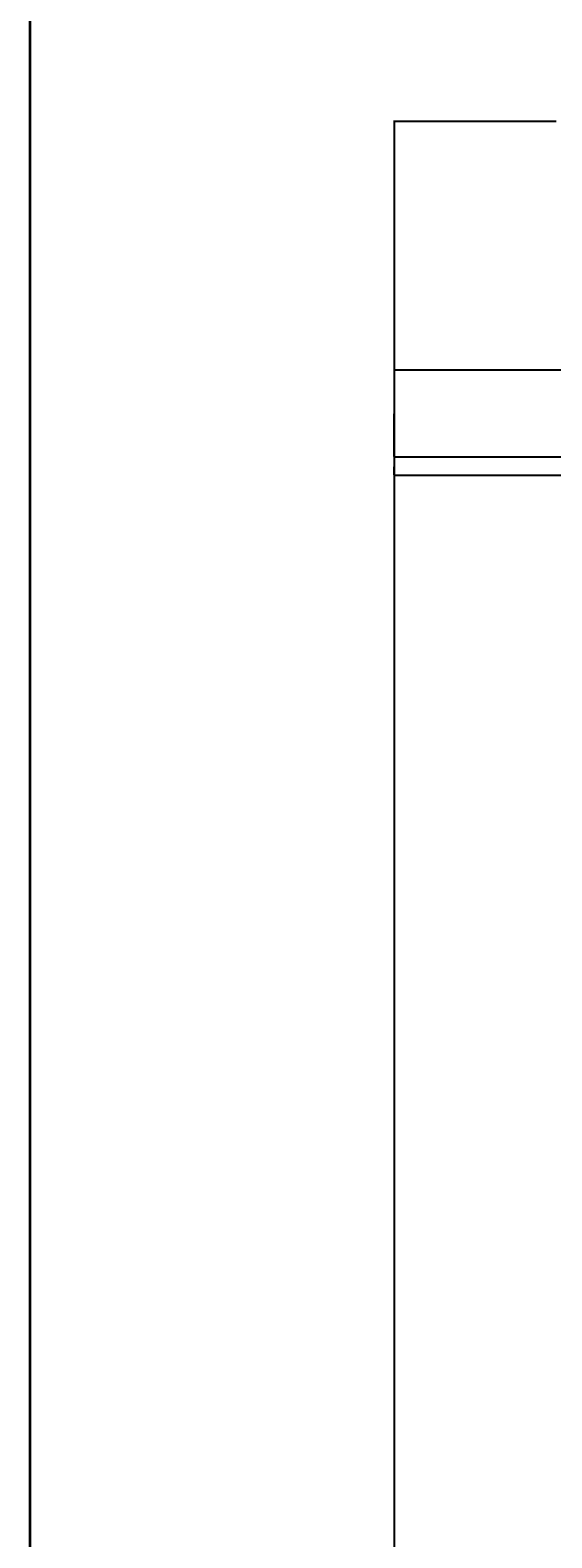
# Model space of a CAD drawing. Units: inches. Extents: x 392 to 1254, y 1207 to 2665.
# Tile 5 of 15: x 392 to 540, y 1827 to 2255. Entities that reach past the tile are written whole.
import ezdxf

# ---------------------------------------------------------------- set-up
doc = ezdxf.new("R2010")
doc.units = ezdxf.units.IN
doc.layers.add('A-ANNO-DIMS', color=2, linetype='Continuous', lineweight=18)
doc.layers.add('A-ANNO-TTLB', color=7, linetype='Continuous', lineweight=35)
doc.styles.get("Standard").update_dxf_attribs({"font": 'arial.ttf'})
doc.dimstyles.get("Standard").update_dxf_attribs({"dimtxt": 0.18, "dimasz": 0.18, "dimexe": 0.18, "dimexo": 0.0625, "dimgap": 0.09, "dimtad": 0, "dimtih": 1, "dimtoh": 1, "dimdec": 4, "dimzin": 0, "dimdsep": 46, "dimtxsty": 'Standard', "dimcen": 0.09, "dimadec": 0, "dimazin": 0, "dimtfac": 1, "dimtdec": 4, "dimtofl": 0, "dimtmove": 0, "dimatfit": 3, "dimfxl": 1, "dimtolj": 1, "dimtzin": 0, "dimarcsym": 0})

# ---------------------------------------------------------------- blocks, each defined once
blk = doc.blocks.new('*D26')
at = {"layer": 'A-ANNO-DIMS', "color": 0, "lineweight": -2, "transparency": 16777216}
for p, q in [((541.22, 2229.3), (495, 2229.3)), ((495.18, 2229.12), (495.18, 1819.98)), ((495.18, 1410.48), (495.18, 1819.61)), ((753.23, 1410.3), (495, 1410.3))]:
    blk.add_line(p, q, dxfattribs=at)
at = {"layer": 'A-ANNO-DIMS', "color": 0, "transparency": 16777216}
for points in [[(495.15, 2229.12), (495.21, 2229.12), (495.18, 2229.3)], [(495.15, 1410.48), (495.21, 1410.48), (495.18, 1410.3)]]:
    blk.add_solid(points, dxfattribs=at)
at = {"layer": 'Defpoints', "color": 0, "transparency": 16777216}
for p in [(495.18, 2229.3), (541.28, 2229.3), (753.29, 1410.3)]:
    blk.add_point(p, dxfattribs=at)
at = {"layer": 'A-ANNO-DIMS', "color": 0, "transparency": 16777216, "insert": (495.18, 1819.8), "char_height": 0.18, "attachment_point": 5}
blk.add_mtext('\\A1;819', dxfattribs=at)
blk = doc.blocks.new('*D81')
at = {"layer": 'A-ANNO-DIMS', "color": 0, "lineweight": -2, "transparency": 16777216}
for p, q in [((689.72, 2158.7), (495, 2158.7)), ((495.18, 2158.52), (495.18, 2146.56)), ((495.18, 2134.24), (495.18, 2146.19)), ((689.72, 2134.06), (495, 2134.06))]:
    blk.add_line(p, q, dxfattribs=at)
at = {"layer": 'A-ANNO-DIMS', "color": 0, "transparency": 16777216}
for points in [[(495.15, 2158.52), (495.21, 2158.52), (495.18, 2158.7)], [(495.15, 2134.24), (495.21, 2134.24), (495.18, 2134.06)]]:
    blk.add_solid(points, dxfattribs=at)
at = {"layer": 'Defpoints', "color": 0, "transparency": 16777216}
for p in [(495.18, 2158.7), (689.78, 2158.7), (689.78, 2134.06)]:
    blk.add_point(p, dxfattribs=at)
at = {"layer": 'A-ANNO-DIMS', "color": 0, "transparency": 16777216, "insert": (495.18, 2146.38), "char_height": 0.18, "attachment_point": 5}
blk.add_mtext('\\A1;24.64', dxfattribs=at)
blk = doc.blocks.new('*D82')
at = {"layer": 'A-ANNO-DIMS', "color": 0, "lineweight": -2, "transparency": 16777216}
for p, q in [((689.72, 2134.06), (495, 2134.06)), ((495.18, 2133.88), (495.18, 2131.61)), ((495.18, 2128.98), (495.18, 2131.24)), ((694.22, 2128.8), (495, 2128.8))]:
    blk.add_line(p, q, dxfattribs=at)
at = {"layer": 'A-ANNO-DIMS', "color": 0, "transparency": 16777216}
for points in [[(495.15, 2133.88), (495.21, 2133.88), (495.18, 2134.06)], [(495.15, 2128.98), (495.21, 2128.98), (495.18, 2128.8)]]:
    blk.add_solid(points, dxfattribs=at)
at = {"layer": 'Defpoints', "color": 0, "transparency": 16777216}
for p in [(495.18, 2134.06), (689.78, 2134.06), (694.28, 2128.8)]:
    blk.add_point(p, dxfattribs=at)
at = {"layer": 'A-ANNO-DIMS', "color": 0, "transparency": 16777216, "insert": (495.18, 2131.43), "char_height": 0.18, "attachment_point": 5}
blk.add_mtext('\\A1;5.26', dxfattribs=at)

msp = doc.modelspace()

# ---------------------------------------------------------------- linework, layer by layer
at = {"layer": 'A-ANNO-TTLB'}
msp.add_lwpolyline([(391.939, 2664.8979), (1253.97, 2664.8979), (1253.97, 1207.2611), (391.939, 1207.2611)], close=True, dxfattribs=at)

# ---------------------------------------------------------------- dimensions: what is measured, and where the dimension line sits
at = {"layer": 'A-ANNO-DIMS'}
for base, p1, p2, override, picture, middle in [((495.1807, 2229.2953), (753.2885, 1410.2953), (541.2807, 2229.2953), {"dimdec": 0, "dimlfac": 1, "dimrnd": 0, "dimzin": 0, "dimdsep": 46, "dimlunit": 2}, '*D26', (495.1807, 1819.7953)), ((495.1807, 2158.6973), (689.7807, 2134.0554), (689.7807, 2158.6973), {"dimdec": 2, "dimlfac": 1, "dimrnd": 0, "dimzin": 0, "dimdsep": 46, "dimlunit": 2}, '*D81', (495.1807, 2146.3764)), ((495.1807, 2134.0554), (694.2807, 2128.7953), (689.7807, 2134.0554), {"dimdec": 2, "dimlfac": 1, "dimrnd": 0, "dimzin": 0, "dimdsep": 46, "dimlunit": 2}, '*D82', (495.1807, 2131.4254))]:
    dim = msp.add_linear_dim(base=base, p1=p1, p2=p2, angle=90, dimstyle='Standard', override=override, dxfattribs=at)
    dim.commit()
    dim.dimension.update_dxf_attribs({"geometry": picture, "text_midpoint": middle})

doc.saveas('drawing.dxf')
